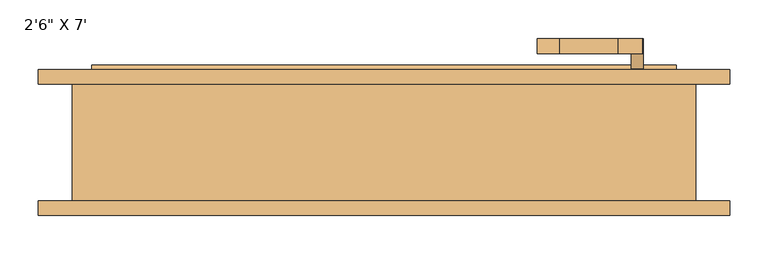
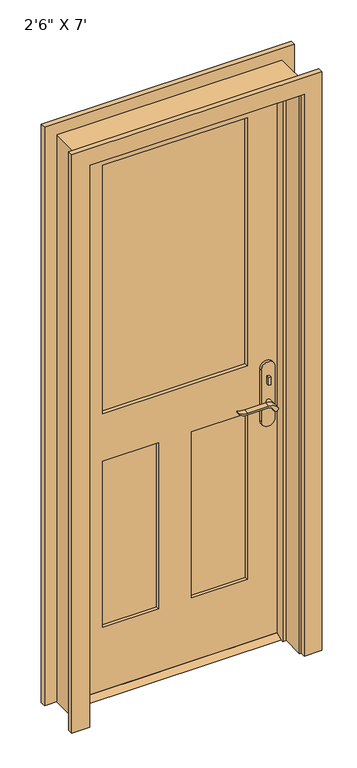
"""IFC4 building model written with IfcOpenShell, lengths in millimetres: door geometry."""

from ifc_helpers import new_model, si_unit, point, frame, frame_2d, origin, place, context, project, spatial, polyline, circle_curve, trimmed, segment, composite_curve, outline, extrude, faceted_brep, source, transform, mapped, element, save


def door_0459eae1(model_context):
    return source(origin(), model_context, "Body", "SolidModel", [
        extrude(outline(polyline([(38.1, 12.7), (73.025, 12.7), (98.425, 0.0), (12.7, 0.0), (38.1, 12.7)])), frame((-381.0, 0.0, 0.0), z_axis=(1.0, 0.0, 0.0), x_axis=(0.0, 1.0, 0.0)), (0.0, 0.0, 1.0), 762.0),
        extrude(outline(polyline([(335.2, 18.1), (325.2, 18.1), (325.2, 28.1), (335.2, 28.1), (335.2, 18.1)])), frame((0.0, 0.0, 981.9), z_axis=(0.0, 0.0, 1.0), x_axis=(1.0, 0.0, 0.0)), (0.0, 0.0, 1.0), 30.0),
        extrude(outline(composite_curve([segment(trimmed(circle_curve(frame_2d((996.9, 330.2)), 8.0), [point((996.9, 322.2))], [point((996.9, 338.2))], False, "CARTESIAN"), True, "CONTINUOUS"), segment(trimmed(circle_curve(frame_2d((996.9, 330.2)), 8.0), [point((996.9, 338.2))], [point((996.9, 322.2))], False, "CARTESIAN"), True, "CONTINUOUS")], self_intersect=False)), frame((0.0, 83.025, 0.0), z_axis=(0.0, 1.0, 0.0), x_axis=(0.0, 0.0, 1.0)), (0.0, 0.0, 1.0), 10.0),
        extrude(outline(composite_curve([segment(trimmed(circle_curve(frame_2d((897.1555521, 306.5324871)), 37.2832219), [point((919.0523287, 336.7081363))], [point((934.4, 304.8325667))], False, "CARTESIAN"), True, "CONTINUOUS"), segment(polyline([(934.4, 304.8325667), (934.4, 228.5564091)]), True, "CONTINUOUS"), segment(trimmed(circle_curve(frame_2d((1017.6850638, 228.6227909)), 83.2850902), [point((934.4, 228.5564091))], [point((939.4, 200.2))], True, "CARTESIAN"), True, "CONTINUOUS"), segment(polyline([(939.4, 200.2), (936.6135558, 200.2)]), True, "CONTINUOUS"), segment(trimmed(circle_curve(frame_2d((986.6709207, 232.1396612)), 59.3791355), [point((936.6135558, 200.2))], [point((927.4, 228.5564091))], False, "CARTESIAN"), True, "CONTINUOUS"), segment(polyline([(927.4, 228.5564091), (927.4, 304.8138099)]), True, "CONTINUOUS"), segment(trimmed(circle_curve(frame_2d((909.2738613, 304.8138099)), 18.1261387), [point((927.4, 304.8138099))], [point((914.4, 322.2))], True, "CARTESIAN"), True, "CONTINUOUS"), segment(trimmed(circle_curve(frame_2d((914.4, 330.2)), 8.0), [point((914.4, 322.2))], [point((919.0523287, 336.7081363))], False, "CARTESIAN"), True, "CONTINUOUS")], self_intersect=False)), frame((0.0, -21.9, 0.0), z_axis=(0.0, 1.0, 0.0), x_axis=(0.0, 0.0, 1.0)), (0.0, 0.0, 1.0), 20.0),
        extrude(outline(composite_curve([segment(trimmed(circle_curve(frame_2d((914.4, 330.2)), 8.0), [point((914.3999903, 322.2))], [point((919.0523287, 336.7081363))], False, "CARTESIAN"), True, "CONTINUOUS"), segment(trimmed(circle_curve(frame_2d((897.1555521, 306.5324871)), 37.2832219), [point((919.0523287, 336.7081363))], [point((934.4, 304.8325667))], False, "CARTESIAN"), True, "CONTINUOUS"), segment(polyline([(934.4, 304.8325667), (934.4, 228.5564091)]), True, "CONTINUOUS"), segment(trimmed(circle_curve(frame_2d((1017.6850638, 228.6227909)), 83.2850902), [point((934.4, 228.5564091))], [point((939.4, 200.2))], True, "CARTESIAN"), True, "CONTINUOUS"), segment(polyline([(939.4, 200.2), (936.6135558, 200.2)]), True, "CONTINUOUS"), segment(trimmed(circle_curve(frame_2d((986.6709207, 232.1396612)), 59.3791355), [point((936.6135558, 200.2))], [point((927.4, 228.5564091))], False, "CARTESIAN"), True, "CONTINUOUS"), segment(polyline([(927.4, 228.5564091), (927.4, 304.8138122)]), True, "CONTINUOUS"), segment(trimmed(circle_curve(frame_2d((909.2738682, 304.8138122)), 18.1261318), [point((927.4, 304.8138122))], [point((914.3999903, 322.2))], True, "CARTESIAN"), True, "CONTINUOUS")], self_intersect=False)), frame((0.0, 113.025, 0.0), z_axis=(0.0, 1.0, 0.0), x_axis=(0.0, 0.0, 1.0)), (0.0, 0.0, 1.0), 20.0),
        extrude(outline(composite_curve([segment(trimmed(circle_curve(frame_2d((914.4, 330.2)), 8.0), [point((914.4, 322.2))], [point((914.4, 338.2))], False, "CARTESIAN"), True, "CONTINUOUS"), segment(trimmed(circle_curve(frame_2d((914.4, 330.2)), 8.0), [point((914.4, 338.2))], [point((914.4, 322.2))], False, "CARTESIAN"), True, "CONTINUOUS")], self_intersect=False)), frame((0.0, -1.9, 0.0), z_axis=(0.0, 1.0, 0.0), x_axis=(0.0, 0.0, 1.0)), (0.0, 0.0, 1.0), 30.0),
        extrude(outline(composite_curve([segment(trimmed(circle_curve(frame_2d((914.4, 330.2)), 8.0), [point((914.4, 322.2))], [point((914.4, 338.2))], False, "CARTESIAN"), True, "CONTINUOUS"), segment(trimmed(circle_curve(frame_2d((914.4, 330.2)), 8.0), [point((914.4, 338.2))], [point((914.4, 322.2))], False, "CARTESIAN"), True, "CONTINUOUS")], self_intersect=False)), frame((0.0, 83.025, 0.0), z_axis=(0.0, 1.0, 0.0), x_axis=(0.0, 0.0, 1.0)), (0.0, 0.0, 1.0), 30.0),
        extrude(outline(composite_curve([segment(polyline([(844.4, 355.2), (1039.4, 355.2)]), True, "CONTINUOUS"), segment(trimmed(circle_curve(frame_2d((1039.4, 330.2)), 25.0), [point((1039.4, 355.2))], [point((1039.4, 305.2))], False, "CARTESIAN"), True, "CONTINUOUS"), segment(polyline([(1039.4, 305.2), (844.4, 305.2)]), True, "CONTINUOUS"), segment(trimmed(circle_curve(frame_2d((844.4, 330.2)), 25.0), [point((844.4, 305.2))], [point((844.4, 355.2))], False, "CARTESIAN"), True, "CONTINUOUS")], self_intersect=False)), frame((0.0, 28.1, 0.0), z_axis=(0.0, 1.0, 0.0), x_axis=(0.0, 0.0, 1.0)), (0.0, 0.0, 1.0), 10.0),
        extrude(outline(composite_curve([segment(polyline([(844.4, 355.2), (1039.4, 355.2)]), True, "CONTINUOUS"), segment(trimmed(circle_curve(frame_2d((1039.4, 330.2)), 25.0), [point((1039.4, 355.2))], [point((1039.4, 305.2))], False, "CARTESIAN"), True, "CONTINUOUS"), segment(polyline([(1039.4, 305.2), (844.4, 305.2)]), True, "CONTINUOUS"), segment(trimmed(circle_curve(frame_2d((844.4, 330.2)), 25.0), [point((844.4, 305.2))], [point((844.4, 355.2))], False, "CARTESIAN"), True, "CONTINUOUS")], self_intersect=False)), frame((0.0, 73.025, 0.0), z_axis=(0.0, 1.0, 0.0), x_axis=(0.0, 0.0, 1.0)), (0.0, 0.0, 1.0), 10.0),
        faceted_brep([(406.4, 73.025, 0.0), (406.4, -79.375, 0.0), (381.0, -79.375, 0.0), (381.0, 3.175, 0.0), (368.3, 3.175, 0.0), (368.3, 38.1, 0.0), (381.0, 38.1, 0.0), (381.0, 73.025, 0.0), (406.4, 73.025, 2159.0), (406.4, -79.375, 2159.0), (-406.4, -79.375, 2159.0), (-406.4, -79.375, 0.0), (-381.0, -79.375, 0.0), (-381.0, -79.375, 2133.6), (381.0, -79.375, 2133.6), (381.0, 3.175, 2133.6), (-381.0, 3.175, 2133.6), (-381.0, 3.175, 0.0), (-368.3, 3.175, 0.0), (-368.3, 3.175, 2120.9), (368.3, 3.175, 2120.9), (368.3, 38.1, 2120.9), (-368.3, 38.1, 2120.9), (-368.3, 38.1, 0.0), (-381.0, 38.1, 0.0), (-381.0, 38.1, 2133.6), (381.0, 38.1, 2133.6), (381.0, 73.025, 2133.6), (-381.0, 73.025, 2133.6), (-381.0, 73.025, 0.0), (-406.4, 73.025, 0.0), (-406.4, 73.025, 2159.0)], [[[0, 1, 2, 3, 4, 5, 6, 7]], [[1, 0, 8, 9]], [[2, 1, 9, 10, 11, 12, 13, 14]], [[3, 2, 14, 15]], [[4, 3, 15, 16, 17, 18, 19, 20]], [[5, 4, 20, 21]], [[6, 5, 21, 22, 23, 24, 25, 26]], [[7, 6, 26, 27]], [[0, 7, 27, 28, 29, 30, 31, 8]], [[9, 8, 31, 10]], [[15, 14, 13, 16]], [[21, 20, 19, 22]], [[27, 26, 25, 28]], [[30, 29, 24, 23, 18, 17, 12, 11]], [[10, 31, 30, 11]], [[16, 13, 12, 17]], [[22, 19, 18, 23]], [[28, 25, 24, 29]]]),
        extrude(outline(polyline([(2133.6, -381.0), (12.7, -381.0), (12.7, 381.0), (2133.6, 381.0), (2133.6, -381.0)]), holes=[polyline([(1066.8, -260.35), (2012.95, -260.35), (2012.95, 260.35), (1066.8, 260.35), (1066.8, -260.35)]), polyline([(885.825, -60.325), (254.0, -60.325), (254.0, -260.35), (885.825, -260.35), (885.825, -60.325)]), polyline([(885.825, 260.35), (254.0, 260.35), (254.0, 60.325), (885.825, 60.325), (885.825, 260.35)])]), frame((0.0, 38.1, 0.0), z_axis=(0.0, 1.0, 0.0), x_axis=(0.0, 0.0, 1.0)), (0.0, 0.0, 1.0), 34.925),
        extrude(outline(polyline([(260.35, 52.07), (-260.35, 52.07), (-260.35, 59.055), (260.35, 59.055), (260.35, 52.07)])), frame((0.0, 0.0, 1066.8), z_axis=(0.0, 0.0, 1.0), x_axis=(1.0, 0.0, 0.0)), (0.0, 0.0, 1.0), 946.15),
        extrude(outline(polyline([(-60.325, 49.7416667), (-260.35, 49.7416667), (-260.35, 61.3833333), (-60.325, 61.3833333), (-60.325, 49.7416667)])), frame((0.0, 0.0, 254.0), z_axis=(0.0, 0.0, 1.0), x_axis=(1.0, 0.0, 0.0)), (0.0, 0.0, 1.0), 631.825),
        extrude(outline(polyline([(260.35, 49.7416667), (60.325, 49.7416667), (60.325, 61.3833333), (260.35, 61.3833333), (260.35, 49.7416667)])), frame((0.0, 0.0, 254.0), z_axis=(0.0, 0.0, 1.0), x_axis=(1.0, 0.0, 0.0)), (0.0, 0.0, 1.0), 631.825),
        extrude(outline(polyline([(0.0, -450.85), (0.0, -387.35), (2139.95, -387.35), (2139.95, 387.35), (0.0, 387.35), (0.0, 450.85), (2203.45, 450.85), (2203.45, -450.85), (0.0, -450.85)])), frame((0.0, 73.025, 0.0), z_axis=(0.0, 1.0, 0.0), x_axis=(0.0, 0.0, 1.0)), (0.0, 0.0, 1.0), 19.05),
        extrude(outline(polyline([(0.0, -450.85), (0.0, -387.35), (2139.95, -387.35), (2139.95, 387.35), (0.0, 387.35), (0.0, 450.85), (2203.45, 450.85), (2203.45, -450.85), (0.0, -450.85)])), frame((0.0, -98.425, 0.0), z_axis=(0.0, 1.0, 0.0), x_axis=(0.0, 0.0, 1.0)), (0.0, 0.0, 1.0), 19.05),
    ])


if __name__ == "__main__":
    model = new_model("IFC4")
    model_context = context("Model", 3, world=origin())
    ifc_project = project(units=[si_unit("LENGTHUNIT", "METRE", prefix="MILLI")], contexts=[model_context])
    site = spatial("IfcSite", under=ifc_project)
    building = spatial("IfcBuilding", under=site)
    placement = place(None, origin())
    door_shape = door_0459eae1(model_context)
    element("IfcDoor", 1, ObjectType="2'6\" X 7'", at=placement, inside=building, context=model_context, shape_type="MappedRepresentation", body=[
        mapped(door_shape, transform((0.0, 0.0, 0.0), x_axis=(1.0, 0.0, 0.0), y_axis=(0.0, 1.0, 0.0), z_axis=(0.0, 0.0, 1.0))),
    ])
    save(model, "model.ifc")

# Revit data of these elements
# Type "2'6\" X 7'"
#   Type Mark = "15"
#   Assembly Code = "B2030100"
#   Analytic Construction = "French door, wood frame with single glass"
#   Top Rail = 0' - 4 3/4"
#   Threshold Offset [instance default] = 0' - 0 1/2"
#   Thickness = 0' - 1 3/8"
#   Thermal Resistance (R) = 1.0696 (h·ft²·°F)/BTU
#   Swing Angle [instance default] = 90.00°
#   Stiles = 0' - 4 3/4"
#   Rough Width = 2' - 8"
#   Rough Height = 7' - 1"
#   Lock Rail = 0' - 7 1/8"
#   Height = 7' - 0"
#   Width = 2' - 6"
#   Heat Transfer Coefficient (U) = 0.9350 BTU/(h·ft²·°F)
#   Door Offset [instance default] = 0' - 0"
#   Bottom Rail = 0' - 9 1/2"
#   Threshold [instance default] = yes
#   Function = 1
#   Exterior Trim [instance default] = yes
#   Trim Material = Cherry
#   Threshold Material = Cherry
#   Panel Material = Cherry
#   Glazing = Glass
#   Frame Material = Cherry
#   Door Handle Material = Aluminum
#   Visual Light Transmittance = 0
#   Solar Heat Gain Coefficient = 0
#   Wall Closure = (empty or 0)
#   Construction Type = (empty or 0)
# Element 1 (IfcDoor, "2'6\" X 7'")
#   Materials on its faces: "Cherry", "Aluminum", "Glass"
# Materials
#   "Cherry": class "Wood", colour RGB 226 177 128, transparency 0, Description = "Prunus Serotina", Cost = 0
#   "Glass": class "Glass", colour RGB 0 128 192, transparency 0.75, Description = "Soda Lime Glass", Cost = 0
#   "Aluminum": class "Metal", colour RGB 247 247 247, transparency 0, Description = "Aluminum 6061", Cost = 0
